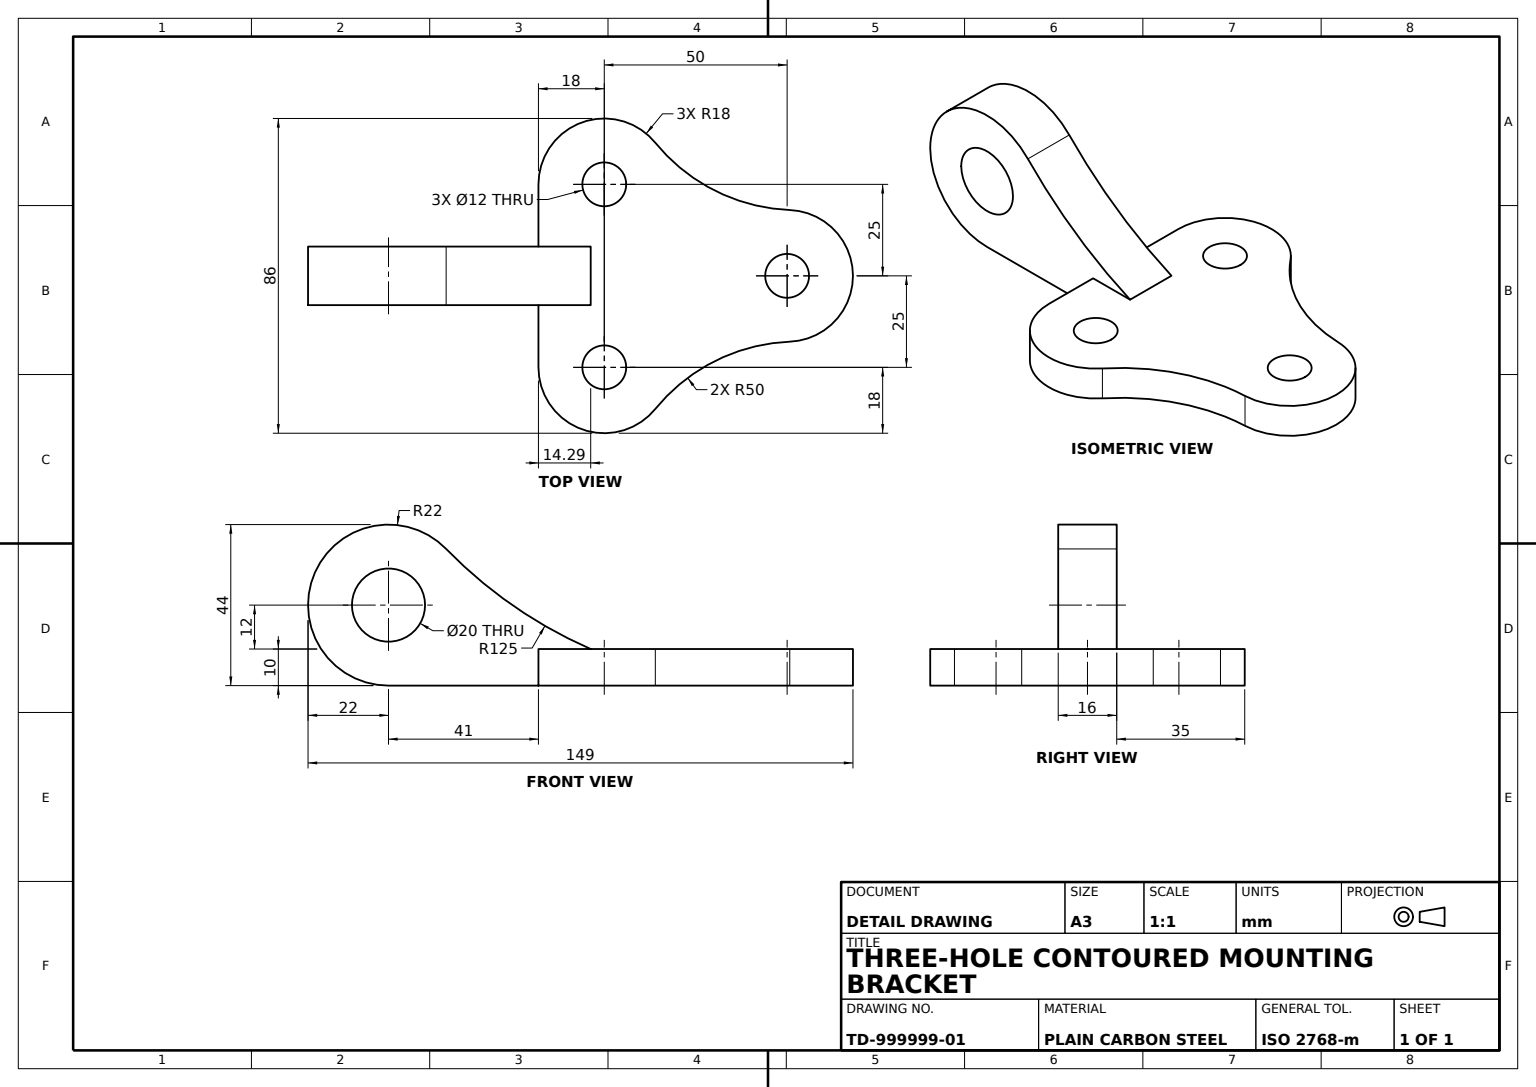
from build123d import *

# Parameters (mm, degrees)
BASE_PLATE_SKETCH_R = 6
BASE_PLATE_DEPTH    = 10
PIVOT_LUG_SKETCH_R  = 10
PIVOT_LUG_DEPTH     = 8


with BuildPart() as part:
    # Base Plate Sketch → Base Plate (new body)
    with BuildSketch(Plane(origin=(0, 0, 0), x_dir=(1, 0, 0), z_dir=(0, 1, 0))):
        with BuildLine():
            Line((25, -68), (8, -68))
            Line((8, -68), (8, -53.71))
            Line((8, -53.71), (-8, -53.71))
            Line((-8, -53.71), (-8, -68))
            Line((-8, -68), (-25, -68))
            ThreePointArc((-25, -68), (-41.958896227, -56.032896381), (-36.367918187, -36.043982083))
            ThreePointArc((-36.367918187, -36.043982083), (-23.224109156, -19.637945422), (-17.985565246, 0.720723799))
            ThreePointArc((-17.985565246, 0.720723799), (0, 18), (17.985565246, 0.720723799))
            ThreePointArc((17.985565246, 0.720723799), (23.224109156, -19.637945422), (36.367918187, -36.043982083))
            ThreePointArc((36.367918187, -36.043982083), (41.958896227, -56.032896381), (25, -68))
        make_face()
        with Locations(Location((0, 0, 0), (0, 0, 270))):
            Circle(BASE_PLATE_SKETCH_R, mode=Mode.SUBTRACT)
        with Locations(Location((-25, -50, 0), (0, 0, 270))):
            Circle(BASE_PLATE_SKETCH_R, mode=Mode.SUBTRACT)
        with Locations(Location((25, -50, 0), (0, 0, 270))):
            Circle(BASE_PLATE_SKETCH_R, mode=Mode.SUBTRACT)
    extrude(amount=BASE_PLATE_DEPTH)

    # Pivot Lug Sketch → Pivot Lug (add, symmetric)
    with BuildSketch(Plane(origin=(0, 0, 0), x_dir=(0, 0, -1), z_dir=(1, 0, 0))):
        with BuildLine():
            Line((-109, 0), (-53.71, 0))
            Line((-53.71, 0), (-53.71, 10))
            ThreePointArc((-53.71, 10), (-74.800840464, 21.756077977), (-93.237910195, 37.347850827))
            ThreePointArc((-93.237910195, 37.347850827), (-129.268851943, 30.554159275), (-109, 0))
        make_face()
        with Locations((-109, 22)):
            Circle(PIVOT_LUG_SKETCH_R, mode=Mode.SUBTRACT)
    extrude(amount=PIVOT_LUG_DEPTH, both=True)


solid = part.part
